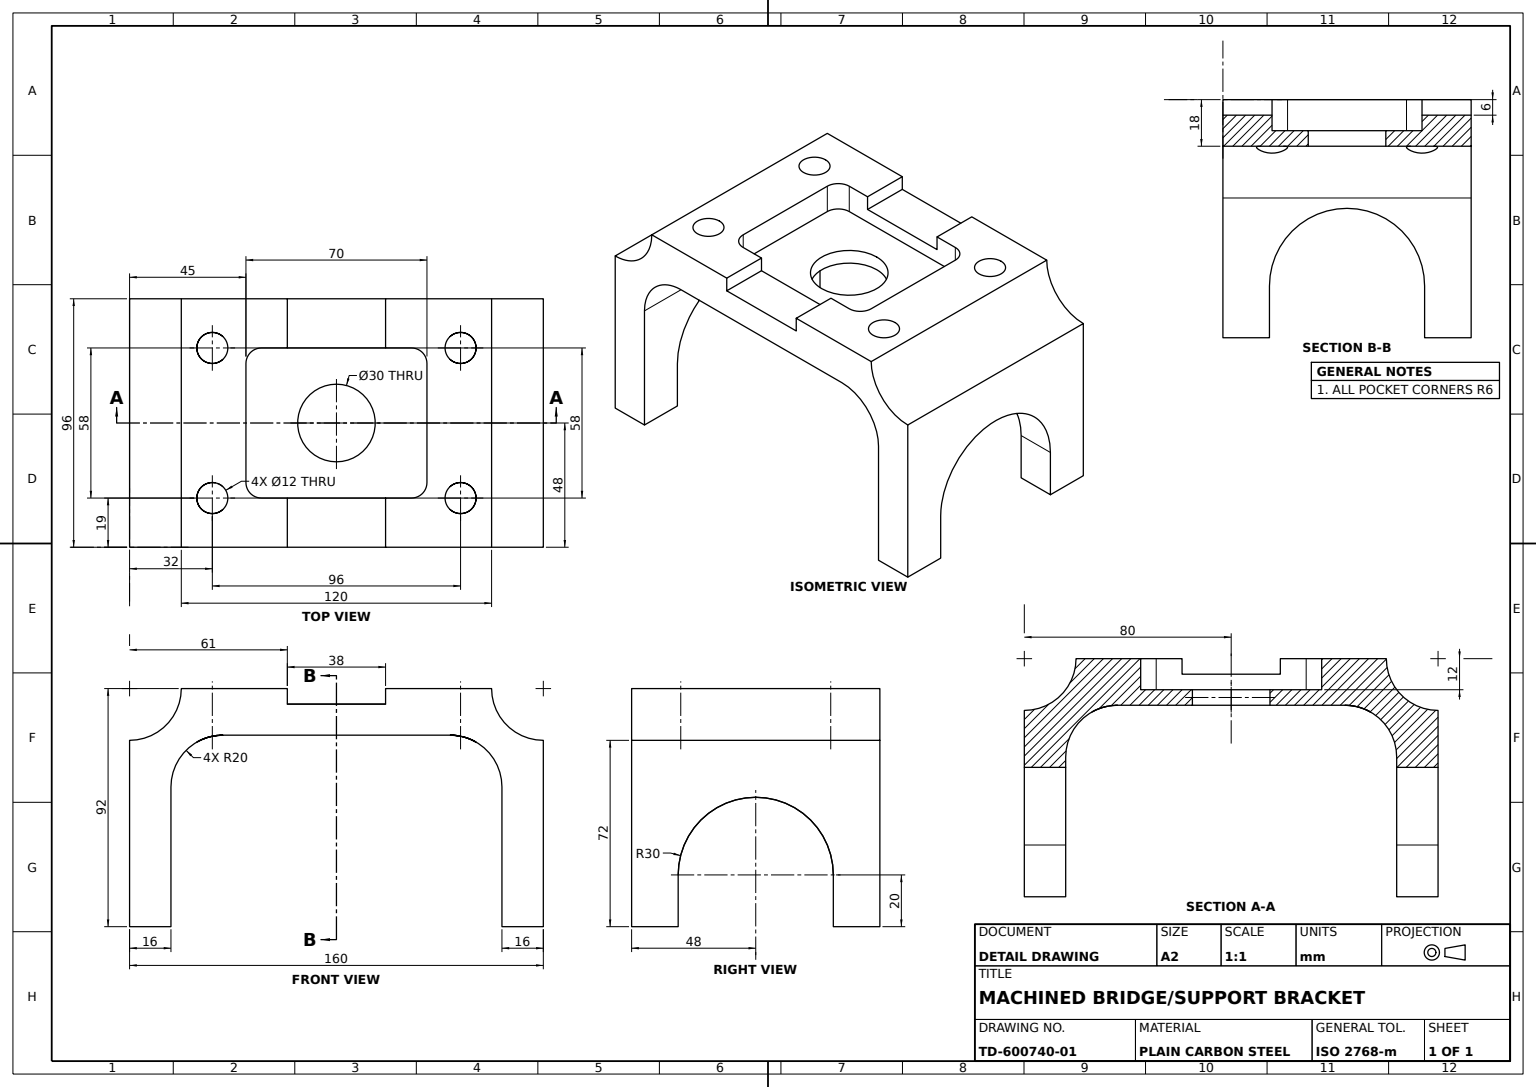
from build123d import *

# Parameters (mm, degrees)
BRIDGE_BODY_DEPTH          = 96
ARCH_RELIEF_CUT_DEPTH      = 209.038457983
TOP_CHANNEL_SKETCH_W       = 38
TOP_CHANNEL_SKETCH_H       = 96
TOP_CHANNEL_38X6_DEPTH     = 6
CENTER_BORE_SKETCH_R       = 15
CENTER_BORE_30_DEPTH       = 152.69706655
MOUNTING_HOLES_SKETCH_R    = 6
MOUNTING_HOLES_4X_12_DEPTH = 156.17731793
CENTER_POCKET_58X70_DEPTH  = 12


with BuildPart() as part:
    # Bridge Profile Sketch → Bridge Body (new body)
    with BuildSketch(Plane.XY):
        with BuildLine():
            Line((-80, 0), (-64, 0))
            Line((-64, 0), (-64, 54))
            ThreePointArc((-64, 54), (-58.142135624, 68.142135624), (-44, 74))
            Line((-44, 74), (44, 74))
            ThreePointArc((44, 74), (58.142135624, 68.142135624), (64, 54))
            Line((64, 54), (64, 0))
            Line((64, 0), (80, 0))
            Line((80, 0), (80, 72))
            ThreePointArc((80, 72), (65.857864376, 77.857864376), (60, 92))
            Line((60, 92), (-60, 92))
            ThreePointArc((-60, 92), (-65.857864376, 77.857864376), (-80, 72))
            Line((-80, 72), (-80, 0))
        make_face()
    extrude(amount=BRIDGE_BODY_DEPTH)

    # Arch Relief Sketch → Arch Relief Cut (cut, through all)
    with BuildSketch(Plane(origin=(80, 0, 0), x_dir=(0, 0, -1), z_dir=(1, 0, 0))):
        with BuildLine():
            Line((-78, 20), (-78, 0))
            Line((-78, 0), (-18, 0))
            Line((-18, 0), (-18, 20))
            ThreePointArc((-18, 20), (-48, 50), (-78, 20))
        make_face()
    extrude(amount=-ARCH_RELIEF_CUT_DEPTH, mode=Mode.SUBTRACT)

    # Top Channel Sketch → Top Channel 38x6 (cut)
    with BuildSketch(Plane(origin=(0, 92, 0), x_dir=(1, 0, 0), z_dir=(0, 1, 0))):
        with Locations((0, -48)):
            Rectangle(TOP_CHANNEL_SKETCH_W, TOP_CHANNEL_SKETCH_H)
    extrude(amount=-TOP_CHANNEL_38X6_DEPTH, mode=Mode.SUBTRACT)

    # Center Bore Sketch → Center Bore Ø30 (cut, through all)
    with BuildSketch(Plane(origin=(0, 86, 0), x_dir=(1, 0, 0), z_dir=(0, 1, 0))):
        with Locations(Location((0, -48, 0), (0, 0, 270))):
            Circle(CENTER_BORE_SKETCH_R)
    extrude(amount=-CENTER_BORE_30_DEPTH, mode=Mode.SUBTRACT)

    # Mounting Holes Sketch → Mounting Holes 4xØ12 (cut, through all)
    with BuildSketch(Plane(origin=(0, 92, 0), x_dir=(1, 0, 0), z_dir=(0, 1, 0))):
        with Locations(Location((-48, -19, 0), (0, 0, 270))):
            Circle(MOUNTING_HOLES_SKETCH_R)
        with Locations(Location((48, -19, 0), (0, 0, 270))):
            Circle(MOUNTING_HOLES_SKETCH_R)
        with Locations(Location((48, -77, 0), (0, 0, 270))):
            Circle(MOUNTING_HOLES_SKETCH_R)
        with Locations(Location((-48, -77, 0), (0, 0, 270))):
            Circle(MOUNTING_HOLES_SKETCH_R)
    extrude(amount=-MOUNTING_HOLES_4X_12_DEPTH, mode=Mode.SUBTRACT)

    # Center Pocket Sketch → Center Pocket 58x70 (cut)
    with BuildSketch(Plane(origin=(0, 92, 0), x_dir=(1, 0, 0), z_dir=(0, 1, 0))):
        with BuildLine():
            Line((-29, -77), (29, -77))
            ThreePointArc((29, -77), (33.242640687, -75.242640687), (35, -71))
            Line((35, -71), (35, -25))
            ThreePointArc((35, -25), (33.242640687, -20.757359313), (29, -19))
            Line((29, -19), (-29, -19))
            ThreePointArc((-29, -19), (-33.242640687, -20.757359313), (-35, -25))
            Line((-35, -25), (-35, -71))
            ThreePointArc((-35, -71), (-33.242640687, -75.242640687), (-29, -77))
        make_face()
    extrude(amount=-CENTER_POCKET_58X70_DEPTH, mode=Mode.SUBTRACT)


solid = part.part
